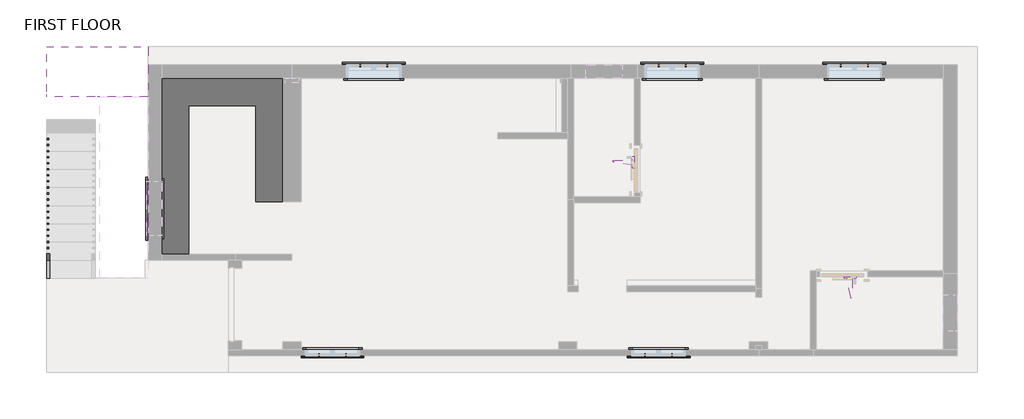
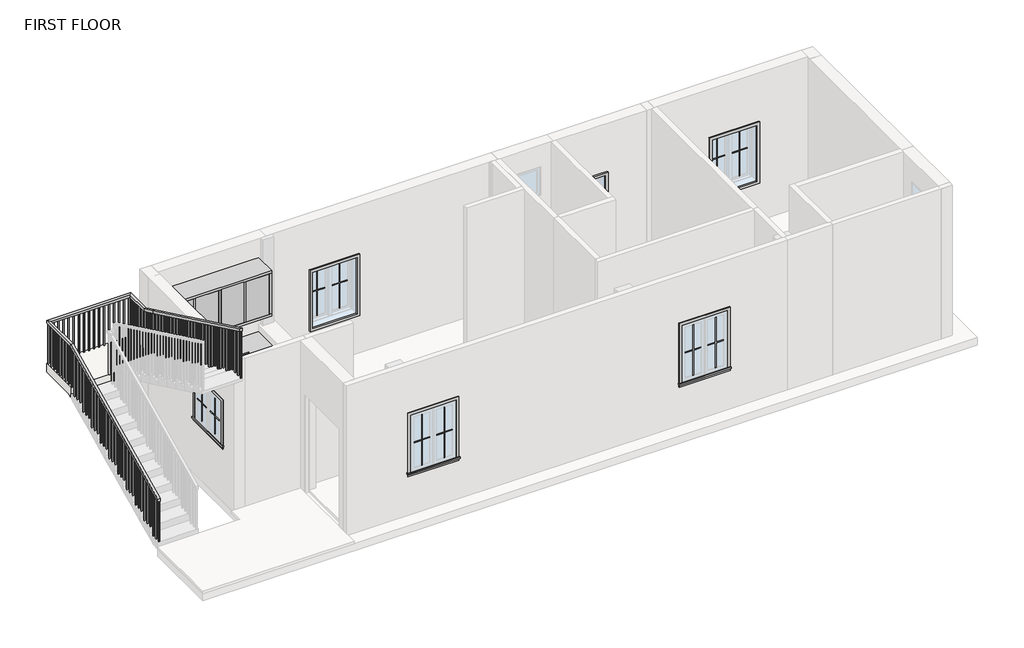
# One storey, part 3 of 3: 27 proxies, 1 railing, 1 slab.
"""IFC4 building model written with IfcOpenShell, lengths in millimetres."""

from ifc_helpers import new_model, si_unit, frame, origin, place, context, project, spatial, polyline, outline, extrude, faceted_brep, transform, mapped, element, save
from components import bel_door_closer_bel_door_closer_f210e2f3, bel_door_closer_bel_door_closer_a3520c2f, generic_models_2_generic_models_1_30118c6b, muntin_pattern_2x2_muntin_pattern_2x2_1acec82f, muntin_pattern_2x2_muntin_pattern_2x2_43d02eee, muntin_pattern_2x2_muntin_pattern_2x2_d1c6e638, muntin_pattern_2x2_muntin_pattern_2x2_37b95fb2, trim_window_exterior_flat_with_sill_e4b28ec3, trim_window_exterior_flat_with_sill_84e24481, trim_window_interior_flat_picture_frame_39ff4276, trim_window_interior_flat_picture_frame_28d4e5dc

model = new_model("IFC4")

# Units and contexts
model_context = context("Model", 3, world=origin())
ifc_project = project(units=[si_unit("LENGTHUNIT", "METRE", prefix="MILLI")], contexts=[model_context])

# Site, building, storey
site = spatial("IfcSite", under=ifc_project)
building = spatial("IfcBuilding", under=site)
storey = spatial("IfcBuildingStorey", under=building, Name="FIRST FLOOR", Elevation=3200.4)

# Proxies
placement = place(None, origin())
bel_door_closer_bel_door_closer_shape = bel_door_closer_bel_door_closer_f210e2f3(model_context)
element("IfcBuildingElementProxy", 1, Name="BEL-Door Closer : BEL-Door Closer", ObjectType="BEL-Door Closer : BEL-Door Closer", at=placement, inside=storey, context=model_context, shape_type="MappedRepresentation", body=[
    mapped(bel_door_closer_bel_door_closer_shape, transform((6826.3533773, 1546.5642852, 5345.0957985), x_axis=(-1.0, 0.0, 0.0), y_axis=(0.0, 0.0, -1.0), z_axis=(0.0, -1.0, 0.0))),
])
bel_door_closer_bel_door_closer_2_shape = bel_door_closer_bel_door_closer_a3520c2f(model_context)
element("IfcBuildingElementProxy", 2, Name="BEL-Door Closer : BEL-Door Closer", ObjectType="BEL-Door Closer : BEL-Door Closer", at=placement, inside=storey, context=model_context, shape_type="MappedRepresentation", body=[
    mapped(bel_door_closer_bel_door_closer_2_shape, transform((3460.0408773, 3211.0767852, 5345.0957985), x_axis=(0.0, -1.0, 0.0), y_axis=(0.0, 0.0, 1.0), z_axis=(-1.0, 0.0, 0.0))),
])
generic_models_2_generic_models_1_shape = generic_models_2_generic_models_1_30118c6b(model_context)
element("IfcBuildingElementProxy", 3, Name="Generic Models 2 : Generic Models 1", ObjectType="Generic Models 2 : Generic Models 1", at=placement, inside=storey, context=model_context, shape_type="MappedRepresentation", body=[
    mapped(generic_models_2_generic_models_1_shape, transform((0.0, 0.0, 0.0), x_axis=(1.0, 0.0, 0.0), y_axis=(0.0, 1.0, 0.0), z_axis=(0.0, 0.0, 1.0))),
])
muntin_pattern_2x2_muntin_pattern_2x2_shape = muntin_pattern_2x2_muntin_pattern_2x2_1acec82f(model_context)
element("IfcBuildingElementProxy", 4, Name="Muntin Pattern_2x2 : Muntin Pattern_2x2", ObjectType="Muntin Pattern_2x2 : Muntin Pattern_2x2", at=placement, inside=storey, context=model_context, shape_type="MappedRepresentation", body=[
    mapped(muntin_pattern_2x2_muntin_pattern_2x2_shape, transform((-1135.7716227, 5093.0392852, 4184.65), x_axis=(1.0, 0.0, 0.0), y_axis=(0.0, 1.0, 0.0), z_axis=(0.0, 0.0, 1.0))),
])
element("IfcBuildingElementProxy", 5, Name="Muntin Pattern_2x2 : Muntin Pattern_2x2", ObjectType="Muntin Pattern_2x2 : Muntin Pattern_2x2", at=placement, inside=storey, context=model_context, shape_type="MappedRepresentation", body=[
    mapped(muntin_pattern_2x2_muntin_pattern_2x2_shape, transform((3868.0283773, 5093.0392852, 4184.65), x_axis=(1.0, 0.0, 0.0), y_axis=(0.0, 1.0, 0.0), z_axis=(0.0, 0.0, 1.0))),
])
element("IfcBuildingElementProxy", 6, Name="Muntin Pattern_2x2 : Muntin Pattern_2x2", ObjectType="Muntin Pattern_2x2 : Muntin Pattern_2x2", at=placement, inside=storey, context=model_context, shape_type="MappedRepresentation", body=[
    mapped(muntin_pattern_2x2_muntin_pattern_2x2_shape, transform((6922.3783773, 5093.0392852, 4184.65), x_axis=(1.0, 0.0, 0.0), y_axis=(0.0, 1.0, 0.0), z_axis=(0.0, 0.0, 1.0))),
])
element("IfcBuildingElementProxy", 7, Name="Muntin Pattern_2x2 : Muntin Pattern_2x2", ObjectType="Muntin Pattern_2x2 : Muntin Pattern_2x2", at=placement, inside=storey, context=model_context, shape_type="MappedRepresentation", body=[
    mapped(muntin_pattern_2x2_muntin_pattern_2x2_shape, transform((4093.4533773, 235.2892852, 4184.65), x_axis=(-1.0, 0.0, 0.0), y_axis=(0.0, -1.0, 0.0), z_axis=(0.0, 0.0, 1.0))),
])
element("IfcBuildingElementProxy", 8, Name="Muntin Pattern_2x2 : Muntin Pattern_2x2", ObjectType="Muntin Pattern_2x2 : Muntin Pattern_2x2", at=placement, inside=storey, context=model_context, shape_type="MappedRepresentation", body=[
    mapped(muntin_pattern_2x2_muntin_pattern_2x2_shape, transform((-1373.8966227, 235.2892852, 4184.65), x_axis=(-1.0, 0.0, 0.0), y_axis=(0.0, -1.0, 0.0), z_axis=(0.0, 0.0, 1.0))),
])
muntin_pattern_2x2_muntin_pattern_2x2_2_shape = muntin_pattern_2x2_muntin_pattern_2x2_43d02eee(model_context)
element("IfcBuildingElementProxy", 9, Name="Muntin Pattern_2x2 : Muntin Pattern_2x2", ObjectType="Muntin Pattern_2x2 : Muntin Pattern_2x2", at=placement, inside=storey, context=model_context, shape_type="MappedRepresentation", body=[
    mapped(muntin_pattern_2x2_muntin_pattern_2x2_2_shape, transform((-681.7466227, 5093.0392852, 4184.65), x_axis=(-1.0, 0.0, 0.0), y_axis=(0.0, -1.0, 0.0), z_axis=(0.0, 0.0, 1.0))),
])
element("IfcBuildingElementProxy", 10, Name="Muntin Pattern_2x2 : Muntin Pattern_2x2", ObjectType="Muntin Pattern_2x2 : Muntin Pattern_2x2", at=placement, inside=storey, context=model_context, shape_type="MappedRepresentation", body=[
    mapped(muntin_pattern_2x2_muntin_pattern_2x2_2_shape, transform((4322.0533773, 5093.0392852, 4184.65), x_axis=(-1.0, 0.0, 0.0), y_axis=(0.0, -1.0, 0.0), z_axis=(0.0, 0.0, 1.0))),
])
element("IfcBuildingElementProxy", 11, Name="Muntin Pattern_2x2 : Muntin Pattern_2x2", ObjectType="Muntin Pattern_2x2 : Muntin Pattern_2x2", at=placement, inside=storey, context=model_context, shape_type="MappedRepresentation", body=[
    mapped(muntin_pattern_2x2_muntin_pattern_2x2_2_shape, transform((7376.4033773, 5093.0392852, 4184.65), x_axis=(-1.0, 0.0, 0.0), y_axis=(0.0, -1.0, 0.0), z_axis=(0.0, 0.0, 1.0))),
])
element("IfcBuildingElementProxy", 12, Name="Muntin Pattern_2x2 : Muntin Pattern_2x2", ObjectType="Muntin Pattern_2x2 : Muntin Pattern_2x2", at=placement, inside=storey, context=model_context, shape_type="MappedRepresentation", body=[
    mapped(muntin_pattern_2x2_muntin_pattern_2x2_2_shape, transform((3639.4283773, 235.2892852, 4184.65), x_axis=(1.0, 0.0, 0.0), y_axis=(0.0, 1.0, 0.0), z_axis=(0.0, 0.0, 1.0))),
])
element("IfcBuildingElementProxy", 13, Name="Muntin Pattern_2x2 : Muntin Pattern_2x2", ObjectType="Muntin Pattern_2x2 : Muntin Pattern_2x2", at=placement, inside=storey, context=model_context, shape_type="MappedRepresentation", body=[
    mapped(muntin_pattern_2x2_muntin_pattern_2x2_2_shape, transform((-1827.9216227, 235.2892852, 4184.65), x_axis=(1.0, 0.0, 0.0), y_axis=(0.0, 1.0, 0.0), z_axis=(0.0, 0.0, 1.0))),
])
muntin_pattern_2x2_muntin_pattern_2x2_3_shape = muntin_pattern_2x2_muntin_pattern_2x2_d1c6e638(model_context)
element("IfcBuildingElementProxy", 14, Name="Muntin Pattern_2x2 : Muntin Pattern_2x2", ObjectType="Muntin Pattern_2x2 : Muntin Pattern_2x2", at=placement, inside=storey, context=model_context, shape_type="MappedRepresentation", body=[
    mapped(muntin_pattern_2x2_muntin_pattern_2x2_3_shape, transform((-4683.8341227, 2462.5517852, 4489.45), x_axis=(0.0, 1.0, 0.0), y_axis=(-1.0, 0.0, 0.0), z_axis=(0.0, 0.0, 1.0))),
])
muntin_pattern_2x2_muntin_pattern_2x2_4_shape = muntin_pattern_2x2_muntin_pattern_2x2_37b95fb2(model_context)
element("IfcBuildingElementProxy", 15, Name="Muntin Pattern_2x2 : Muntin Pattern_2x2", ObjectType="Muntin Pattern_2x2 : Muntin Pattern_2x2", at=placement, inside=storey, context=model_context, shape_type="MappedRepresentation", body=[
    mapped(muntin_pattern_2x2_muntin_pattern_2x2_4_shape, transform((-4683.8341227, 2916.5767852, 4489.45), x_axis=(0.0, -1.0, 0.0), y_axis=(1.0, 0.0, 0.0), z_axis=(0.0, 0.0, 1.0))),
])
trim_window_exterior_flat_with_sill_shape = trim_window_exterior_flat_with_sill_e4b28ec3(model_context)
element("IfcBuildingElementProxy", 16, Name="Trim-Window-Exterior-Flat : with Sill", ObjectType="Trim-Window-Exterior-Flat : with Sill", at=placement, inside=storey, context=model_context, shape_type="MappedRepresentation", body=[
    mapped(trim_window_exterior_flat_with_sill_shape, transform((-908.7591227, 5102.5642852, 5334.0), x_axis=(-1.0, 0.0, 0.0), y_axis=(0.0, 0.0, 1.0), z_axis=(0.0, 1.0, 0.0))),
])
element("IfcBuildingElementProxy", 17, Name="Trim-Window-Exterior-Flat : with Sill", ObjectType="Trim-Window-Exterior-Flat : with Sill", at=placement, inside=storey, context=model_context, shape_type="MappedRepresentation", body=[
    mapped(trim_window_exterior_flat_with_sill_shape, transform((4095.0408773, 5102.5642852, 5334.0), x_axis=(-1.0, 0.0, 0.0), y_axis=(0.0, 0.0, 1.0), z_axis=(0.0, 1.0, 0.0))),
])
element("IfcBuildingElementProxy", 18, Name="Trim-Window-Exterior-Flat : with Sill", ObjectType="Trim-Window-Exterior-Flat : with Sill", at=placement, inside=storey, context=model_context, shape_type="MappedRepresentation", body=[
    mapped(trim_window_exterior_flat_with_sill_shape, transform((7149.3908773, 5102.5642852, 5334.0), x_axis=(-1.0, 0.0, 0.0), y_axis=(0.0, 0.0, 1.0), z_axis=(0.0, 1.0, 0.0))),
])
element("IfcBuildingElementProxy", 19, Name="Trim-Window-Exterior-Flat : with Sill", ObjectType="Trim-Window-Exterior-Flat : with Sill", at=placement, inside=storey, context=model_context, shape_type="MappedRepresentation", body=[
    mapped(trim_window_exterior_flat_with_sill_shape, transform((3866.4408773, 225.7642852, 5334.0), x_axis=(1.0, 0.0, 0.0), y_axis=(0.0, 0.0, 1.0), z_axis=(0.0, -1.0, 0.0))),
])
element("IfcBuildingElementProxy", 20, Name="Trim-Window-Exterior-Flat : with Sill", ObjectType="Trim-Window-Exterior-Flat : with Sill", at=placement, inside=storey, context=model_context, shape_type="MappedRepresentation", body=[
    mapped(trim_window_exterior_flat_with_sill_shape, transform((-1600.9091227, 225.7642852, 5334.0), x_axis=(1.0, 0.0, 0.0), y_axis=(0.0, 0.0, 1.0), z_axis=(0.0, -1.0, 0.0))),
])
trim_window_exterior_flat_with_sill_2_shape = trim_window_exterior_flat_with_sill_84e24481(model_context)
element("IfcBuildingElementProxy", 21, Name="Trim-Window-Exterior-Flat : with Sill", ObjectType="Trim-Window-Exterior-Flat : with Sill", at=placement, inside=storey, context=model_context, shape_type="MappedRepresentation", body=[
    mapped(trim_window_exterior_flat_with_sill_2_shape, transform((-4693.3591227, 2689.5642852, 5334.0), x_axis=(0.0, -1.0, 0.0), y_axis=(0.0, 0.0, 1.0), z_axis=(-1.0, 0.0, 0.0))),
])
trim_window_interior_flat_picture_frame_shape = trim_window_interior_flat_picture_frame_39ff4276(model_context)
element("IfcBuildingElementProxy", 22, Name="Trim-Window-Interior-Flat : Picture Frame", ObjectType="Trim-Window-Interior-Flat : Picture Frame", at=placement, inside=storey, context=model_context, shape_type="MappedRepresentation", body=[
    mapped(trim_window_interior_flat_picture_frame_shape, transform((-908.7591227, 4873.9642852, 5334.0), x_axis=(1.0, 0.0, 0.0), y_axis=(0.0, 0.0, 1.0), z_axis=(0.0, -1.0, 0.0))),
])
element("IfcBuildingElementProxy", 23, Name="Trim-Window-Interior-Flat : Picture Frame", ObjectType="Trim-Window-Interior-Flat : Picture Frame", at=placement, inside=storey, context=model_context, shape_type="MappedRepresentation", body=[
    mapped(trim_window_interior_flat_picture_frame_shape, transform((4095.0408773, 4873.9642852, 5334.0), x_axis=(1.0, 0.0, 0.0), y_axis=(0.0, 0.0, 1.0), z_axis=(0.0, -1.0, 0.0))),
])
element("IfcBuildingElementProxy", 24, Name="Trim-Window-Interior-Flat : Picture Frame", ObjectType="Trim-Window-Interior-Flat : Picture Frame", at=placement, inside=storey, context=model_context, shape_type="MappedRepresentation", body=[
    mapped(trim_window_interior_flat_picture_frame_shape, transform((7149.3908773, 4873.9642852, 5334.0), x_axis=(1.0, 0.0, 0.0), y_axis=(0.0, 0.0, 1.0), z_axis=(0.0, -1.0, 0.0))),
])
element("IfcBuildingElementProxy", 25, Name="Trim-Window-Interior-Flat : Picture Frame", ObjectType="Trim-Window-Interior-Flat : Picture Frame", at=placement, inside=storey, context=model_context, shape_type="MappedRepresentation", body=[
    mapped(trim_window_interior_flat_picture_frame_shape, transform((3866.4408773, 327.3642852, 5334.0), x_axis=(-1.0, 0.0, 0.0), y_axis=(0.0, 0.0, 1.0), z_axis=(0.0, 1.0, 0.0))),
])
element("IfcBuildingElementProxy", 26, Name="Trim-Window-Interior-Flat : Picture Frame", ObjectType="Trim-Window-Interior-Flat : Picture Frame", at=placement, inside=storey, context=model_context, shape_type="MappedRepresentation", body=[
    mapped(trim_window_interior_flat_picture_frame_shape, transform((-1600.9091227, 327.3642852, 5334.0), x_axis=(-1.0, 0.0, 0.0), y_axis=(0.0, 0.0, 1.0), z_axis=(0.0, 1.0, 0.0))),
])
trim_window_interior_flat_picture_frame_2_shape = trim_window_interior_flat_picture_frame_28d4e5dc(model_context)
element("IfcBuildingElementProxy", 27, Name="Trim-Window-Interior-Flat : Picture Frame", ObjectType="Trim-Window-Interior-Flat : Picture Frame", at=placement, inside=storey, context=model_context, shape_type="MappedRepresentation", body=[
    mapped(trim_window_interior_flat_picture_frame_2_shape, transform((-4464.7591227, 2689.5642852, 5334.0), x_axis=(0.0, 1.0, 0.0), y_axis=(0.0, 0.0, 1.0), z_axis=(1.0, 0.0, 0.0))),
])

# Railing
element("IfcRailing", 28, ObjectType="Handrail - Rectangular", at=placement, inside=storey, context=model_context, shape_type="SolidModel", body=[
    faceted_brep([(-6395.1591227, 1521.1642852, 4260.2727273), (-6395.1591227, 1521.1642852, 4203.9834559), (-6344.3591227, 1521.1642852, 4203.9834559), (-6344.3591227, 1521.1642852, 4260.2727273), (-6395.1591227, 4569.1642852, 5715.0), (-6395.1591227, 4580.6656156, 5664.2), (-6344.3591227, 4580.6656156, 5664.2), (-6344.3591227, 4569.1642852, 5715.0), (-6395.1591227, 5407.3642852, 5715.0), (-6395.1591227, 5407.3642852, 5664.2), (-6344.3591227, 5356.5642852, 5664.2), (-6344.3591227, 5356.5642852, 5715.0), (-4693.3591227, 5407.3642852, 5715.0), (-4693.3591227, 5407.3642852, 5664.2), (-4744.1591227, 5356.5642852, 5664.2), (-4744.1591227, 5356.5642852, 5715.0), (-4693.3591227, 4873.9642852, 5715.0), (-4693.3591227, 4862.4629548, 5664.2), (-4744.1591227, 4862.4629548, 5664.2), (-4744.1591227, 4873.9642852, 5715.0), (-4693.3591227, 4569.1642852, 5860.4727273), (-4693.3591227, 4547.2832222, 5814.6266906), (-4744.1591227, 4547.2832222, 5814.6266906), (-4744.1591227, 4569.1642852, 5860.4727273), (-4693.3591227, 1521.1642852, 7315.2), (-4744.1591227, 1521.1642852, 7315.2), (-4744.1591227, 1521.1642852, 7258.9107287), (-4693.3591227, 1521.1642852, 7258.9107287)], [[[0, 1, 2, 3]], [[1, 0, 4, 5]], [[2, 1, 5, 6]], [[3, 2, 6, 7]], [[0, 3, 7, 4]], [[5, 4, 8, 9]], [[6, 5, 9, 10]], [[7, 6, 10, 11]], [[4, 7, 11, 8]], [[9, 8, 12, 13]], [[10, 9, 13, 14]], [[11, 10, 14, 15]], [[8, 11, 15, 12]], [[13, 12, 16, 17]], [[14, 13, 17, 18]], [[15, 14, 18, 19]], [[12, 15, 19, 16]], [[17, 16, 20, 21]], [[18, 17, 21, 22]], [[19, 18, 22, 23]], [[16, 19, 23, 20]], [[24, 25, 26, 27]], [[21, 20, 24, 27]], [[22, 21, 27, 26]], [[23, 22, 26, 25]], [[20, 23, 25, 24]]]),
    extrude(outline(polyline([(1632.2892852, 7205.8737969), (1632.2892852, 6255.3272727), (1613.2392852, 6255.3272727), (1613.2392852, 7214.9658423), (1632.2892852, 7205.8737969)])), frame((-4728.2841227, 0.0, 0.0), z_axis=(1.0, 0.0, 0.0), x_axis=(0.0, 1.0, 0.0)), (0.0, 0.0, 1.0), 19.05),
    extrude(outline(polyline([(1733.8892852, 7157.3828878), (1733.8892852, 6255.3272727), (1714.8392852, 6255.3272727), (1714.8392852, 7166.4749332), (1733.8892852, 7157.3828878)])), frame((-4728.2841227, 0.0, 0.0), z_axis=(1.0, 0.0, 0.0), x_axis=(0.0, 1.0, 0.0)), (0.0, 0.0, 1.0), 19.05),
    extrude(outline(polyline([(1835.4892852, 7108.8919787), (1835.4892852, 6255.3272727), (1816.4392852, 6255.3272727), (1816.4392852, 7117.9840241), (1835.4892852, 7108.8919787)])), frame((-4728.2841227, 0.0, 0.0), z_axis=(1.0, 0.0, 0.0), x_axis=(0.0, 1.0, 0.0)), (0.0, 0.0, 1.0), 19.05),
    extrude(outline(polyline([(1937.0892852, 7060.4010696), (1937.0892852, 6109.8545455), (1918.0392852, 6109.8545455), (1918.0392852, 7069.493115), (1937.0892852, 7060.4010696)])), frame((-4728.2841227, 0.0, 0.0), z_axis=(1.0, 0.0, 0.0), x_axis=(0.0, 1.0, 0.0)), (0.0, 0.0, 1.0), 19.05),
    extrude(outline(polyline([(2038.6892852, 7011.9101605), (2038.6892852, 6109.8545455), (2019.6392852, 6109.8545455), (2019.6392852, 7021.0022059), (2038.6892852, 7011.9101605)])), frame((-4728.2841227, 0.0, 0.0), z_axis=(1.0, 0.0, 0.0), x_axis=(0.0, 1.0, 0.0)), (0.0, 0.0, 1.0), 19.05),
    extrude(outline(polyline([(2140.2892852, 6963.4192514), (2140.2892852, 6109.8545455), (2121.2392852, 6109.8545455), (2121.2392852, 6972.5112969), (2140.2892852, 6963.4192514)])), frame((-4728.2841227, 0.0, 0.0), z_axis=(1.0, 0.0, 0.0), x_axis=(0.0, 1.0, 0.0)), (0.0, 0.0, 1.0), 19.05),
    extrude(outline(polyline([(2241.8892852, 6914.9283423), (2241.8892852, 5964.3818182), (2222.8392852, 5964.3818182), (2222.8392852, 6924.0203878), (2241.8892852, 6914.9283423)])), frame((-4728.2841227, 0.0, 0.0), z_axis=(1.0, 0.0, 0.0), x_axis=(0.0, 1.0, 0.0)), (0.0, 0.0, 1.0), 19.05),
    extrude(outline(polyline([(2343.4892852, 6866.4374332), (2343.4892852, 5964.3818182), (2324.4392852, 5964.3818182), (2324.4392852, 6875.5294787), (2343.4892852, 6866.4374332)])), frame((-4728.2841227, 0.0, 0.0), z_axis=(1.0, 0.0, 0.0), x_axis=(0.0, 1.0, 0.0)), (0.0, 0.0, 1.0), 19.05),
    extrude(outline(polyline([(2445.0892852, 6817.9465241), (2445.0892852, 5964.3818182), (2426.0392852, 5964.3818182), (2426.0392852, 6827.0385696), (2445.0892852, 6817.9465241)])), frame((-4728.2841227, 0.0, 0.0), z_axis=(1.0, 0.0, 0.0), x_axis=(0.0, 1.0, 0.0)), (0.0, 0.0, 1.0), 19.05),
    extrude(outline(polyline([(2546.6892852, 6769.455615), (2546.6892852, 5818.9090909), (2527.6392852, 5818.9090909), (2527.6392852, 6778.5476605), (2546.6892852, 6769.455615)])), frame((-4728.2841227, 0.0, 0.0), z_axis=(1.0, 0.0, 0.0), x_axis=(0.0, 1.0, 0.0)), (0.0, 0.0, 1.0), 19.05),
    extrude(outline(polyline([(2648.2892852, 6720.9647059), (2648.2892852, 5818.9090909), (2629.2392852, 5818.9090909), (2629.2392852, 6730.0567514), (2648.2892852, 6720.9647059)])), frame((-4728.2841227, 0.0, 0.0), z_axis=(1.0, 0.0, 0.0), x_axis=(0.0, 1.0, 0.0)), (0.0, 0.0, 1.0), 19.05),
    extrude(outline(polyline([(2749.8892852, 6672.4737969), (2749.8892852, 5818.9090909), (2730.8392852, 5818.9090909), (2730.8392852, 6681.5658423), (2749.8892852, 6672.4737969)])), frame((-4728.2841227, 0.0, 0.0), z_axis=(1.0, 0.0, 0.0), x_axis=(0.0, 1.0, 0.0)), (0.0, 0.0, 1.0), 19.05),
    extrude(outline(polyline([(2851.4892852, 6623.9828878), (2851.4892852, 5673.4363636), (2832.4392852, 5673.4363636), (2832.4392852, 6633.0749332), (2851.4892852, 6623.9828878)])), frame((-4728.2841227, 0.0, 0.0), z_axis=(1.0, 0.0, 0.0), x_axis=(0.0, 1.0, 0.0)), (0.0, 0.0, 1.0), 19.05),
    extrude(outline(polyline([(2953.0892852, 6575.4919787), (2953.0892852, 5673.4363636), (2934.0392852, 5673.4363636), (2934.0392852, 6584.5840241), (2953.0892852, 6575.4919787)])), frame((-4728.2841227, 0.0, 0.0), z_axis=(1.0, 0.0, 0.0), x_axis=(0.0, 1.0, 0.0)), (0.0, 0.0, 1.0), 19.05),
    extrude(outline(polyline([(3054.6892852, 6527.0010696), (3054.6892852, 5673.4363636), (3035.6392852, 5673.4363636), (3035.6392852, 6536.093115), (3054.6892852, 6527.0010696)])), frame((-4728.2841227, 0.0, 0.0), z_axis=(1.0, 0.0, 0.0), x_axis=(0.0, 1.0, 0.0)), (0.0, 0.0, 1.0), 19.05),
    extrude(outline(polyline([(3156.2892852, 6478.5101605), (3156.2892852, 5527.9636364), (3137.2392852, 5527.9636364), (3137.2392852, 6487.6022059), (3156.2892852, 6478.5101605)])), frame((-4728.2841227, 0.0, 0.0), z_axis=(1.0, 0.0, 0.0), x_axis=(0.0, 1.0, 0.0)), (0.0, 0.0, 1.0), 19.05),
    extrude(outline(polyline([(3257.8892852, 6430.0192514), (3257.8892852, 5527.9636364), (3238.8392852, 5527.9636364), (3238.8392852, 6439.1112969), (3257.8892852, 6430.0192514)])), frame((-4728.2841227, 0.0, 0.0), z_axis=(1.0, 0.0, 0.0), x_axis=(0.0, 1.0, 0.0)), (0.0, 0.0, 1.0), 19.05),
    extrude(outline(polyline([(3359.4892852, 6381.5283423), (3359.4892852, 5527.9636364), (3340.4392852, 5527.9636364), (3340.4392852, 6390.6203878), (3359.4892852, 6381.5283423)])), frame((-4728.2841227, 0.0, 0.0), z_axis=(1.0, 0.0, 0.0), x_axis=(0.0, 1.0, 0.0)), (0.0, 0.0, 1.0), 19.05),
    extrude(outline(polyline([(3461.0892852, 6333.0374332), (3461.0892852, 5382.4909091), (3442.0392852, 5382.4909091), (3442.0392852, 6342.1294787), (3461.0892852, 6333.0374332)])), frame((-4728.2841227, 0.0, 0.0), z_axis=(1.0, 0.0, 0.0), x_axis=(0.0, 1.0, 0.0)), (0.0, 0.0, 1.0), 19.05),
    extrude(outline(polyline([(3562.6892852, 6284.5465241), (3562.6892852, 5382.4909091), (3543.6392852, 5382.4909091), (3543.6392852, 6293.6385696), (3562.6892852, 6284.5465241)])), frame((-4728.2841227, 0.0, 0.0), z_axis=(1.0, 0.0, 0.0), x_axis=(0.0, 1.0, 0.0)), (0.0, 0.0, 1.0), 19.05),
    extrude(outline(polyline([(3664.2892852, 6236.055615), (3664.2892852, 5382.4909091), (3645.2392852, 5382.4909091), (3645.2392852, 6245.1476605), (3664.2892852, 6236.055615)])), frame((-4728.2841227, 0.0, 0.0), z_axis=(1.0, 0.0, 0.0), x_axis=(0.0, 1.0, 0.0)), (0.0, 0.0, 1.0), 19.05),
    extrude(outline(polyline([(3765.8892852, 6187.5647059), (3765.8892852, 5237.0181818), (3746.8392852, 5237.0181818), (3746.8392852, 6196.6567514), (3765.8892852, 6187.5647059)])), frame((-4728.2841227, 0.0, 0.0), z_axis=(1.0, 0.0, 0.0), x_axis=(0.0, 1.0, 0.0)), (0.0, 0.0, 1.0), 19.05),
    extrude(outline(polyline([(3867.4892852, 6139.0737969), (3867.4892852, 5237.0181818), (3848.4392852, 5237.0181818), (3848.4392852, 6148.1658423), (3867.4892852, 6139.0737969)])), frame((-4728.2841227, 0.0, 0.0), z_axis=(1.0, 0.0, 0.0), x_axis=(0.0, 1.0, 0.0)), (0.0, 0.0, 1.0), 19.05),
    extrude(outline(polyline([(3969.0892852, 6090.5828878), (3969.0892852, 5237.0181818), (3950.0392852, 5237.0181818), (3950.0392852, 6099.6749332), (3969.0892852, 6090.5828878)])), frame((-4728.2841227, 0.0, 0.0), z_axis=(1.0, 0.0, 0.0), x_axis=(0.0, 1.0, 0.0)), (0.0, 0.0, 1.0), 19.05),
    extrude(outline(polyline([(4070.6892852, 6042.0919787), (4070.6892852, 5091.5454545), (4051.6392852, 5091.5454545), (4051.6392852, 6051.1840241), (4070.6892852, 6042.0919787)])), frame((-4728.2841227, 0.0, 0.0), z_axis=(1.0, 0.0, 0.0), x_axis=(0.0, 1.0, 0.0)), (0.0, 0.0, 1.0), 19.05),
    extrude(outline(polyline([(4172.2892852, 5993.6010696), (4172.2892852, 5091.5454545), (4153.2392852, 5091.5454545), (4153.2392852, 6002.693115), (4172.2892852, 5993.6010696)])), frame((-4728.2841227, 0.0, 0.0), z_axis=(1.0, 0.0, 0.0), x_axis=(0.0, 1.0, 0.0)), (0.0, 0.0, 1.0), 19.05),
    extrude(outline(polyline([(4273.8892852, 5945.1101605), (4273.8892852, 5091.5454545), (4254.8392852, 5091.5454545), (4254.8392852, 5954.2022059), (4273.8892852, 5945.1101605)])), frame((-4728.2841227, 0.0, 0.0), z_axis=(1.0, 0.0, 0.0), x_axis=(0.0, 1.0, 0.0)), (0.0, 0.0, 1.0), 19.05),
    extrude(outline(polyline([(4375.4892852, 5896.6192514), (4375.4892852, 4946.0727273), (4356.4392852, 4946.0727273), (4356.4392852, 5905.7112969), (4375.4892852, 5896.6192514)])), frame((-4728.2841227, 0.0, 0.0), z_axis=(1.0, 0.0, 0.0), x_axis=(0.0, 1.0, 0.0)), (0.0, 0.0, 1.0), 19.05),
    extrude(outline(polyline([(4477.0892852, 5848.1283423), (4477.0892852, 4946.0727273), (4458.0392852, 4946.0727273), (4458.0392852, 5857.2203878), (4477.0892852, 5848.1283423)])), frame((-4728.2841227, 0.0, 0.0), z_axis=(1.0, 0.0, 0.0), x_axis=(0.0, 1.0, 0.0)), (0.0, 0.0, 1.0), 19.05),
    extrude(outline(polyline([(4680.2892852, 5751.1465241), (4680.2892852, 4800.6), (4661.2392852, 4800.6), (4661.2392852, 5760.2385696), (4680.2892852, 5751.1465241)])), frame((-4728.2841227, 0.0, 0.0), z_axis=(1.0, 0.0, 0.0), x_axis=(0.0, 1.0, 0.0)), (0.0, 0.0, 1.0), 19.05),
    extrude(outline(polyline([(4781.8892852, 5702.655615), (4781.8892852, 4800.6), (4762.8392852, 4800.6), (4762.8392852, 5711.7476605), (4781.8892852, 5702.655615)])), frame((-4728.2841227, 0.0, 0.0), z_axis=(1.0, 0.0, 0.0), x_axis=(0.0, 1.0, 0.0)), (0.0, 0.0, 1.0), 19.05),
    extrude(outline(polyline([(-4709.2341227, 4883.4892852), (-4709.2341227, 4864.4392852), (-4728.2841227, 4864.4392852), (-4728.2841227, 4883.4892852), (-4709.2341227, 4883.4892852)])), frame((0.0, 0.0, 4800.6), z_axis=(0.0, 0.0, 1.0), x_axis=(1.0, 0.0, 0.0)), (0.0, 0.0, 1.0), 863.6),
    extrude(outline(polyline([(-4709.2341227, 4985.0892852), (-4709.2341227, 4966.0392852), (-4728.2841227, 4966.0392852), (-4728.2841227, 4985.0892852), (-4709.2341227, 4985.0892852)])), frame((0.0, 0.0, 4800.6), z_axis=(0.0, 0.0, 1.0), x_axis=(1.0, 0.0, 0.0)), (0.0, 0.0, 1.0), 863.6),
    extrude(outline(polyline([(-4709.2341227, 5086.6892852), (-4709.2341227, 5067.6392852), (-4728.2841227, 5067.6392852), (-4728.2841227, 5086.6892852), (-4709.2341227, 5086.6892852)])), frame((0.0, 0.0, 4800.6), z_axis=(0.0, 0.0, 1.0), x_axis=(1.0, 0.0, 0.0)), (0.0, 0.0, 1.0), 863.6),
    extrude(outline(polyline([(-4709.2341227, 5188.2892852), (-4709.2341227, 5169.2392852), (-4728.2841227, 5169.2392852), (-4728.2841227, 5188.2892852), (-4709.2341227, 5188.2892852)])), frame((0.0, 0.0, 4800.6), z_axis=(0.0, 0.0, 1.0), x_axis=(1.0, 0.0, 0.0)), (0.0, 0.0, 1.0), 863.6),
    extrude(outline(polyline([(-4709.2341227, 5289.8892852), (-4709.2341227, 5270.8392852), (-4728.2841227, 5270.8392852), (-4728.2841227, 5289.8892852), (-4709.2341227, 5289.8892852)])), frame((0.0, 0.0, 4800.6), z_axis=(0.0, 0.0, 1.0), x_axis=(1.0, 0.0, 0.0)), (0.0, 0.0, 1.0), 863.6),
    extrude(outline(polyline([(-4753.6841227, 5391.4892852), (-4734.6341227, 5391.4892852), (-4734.6341227, 5372.4392852), (-4753.6841227, 5372.4392852), (-4753.6841227, 5391.4892852)])), frame((0.0, 0.0, 4800.6), z_axis=(0.0, 0.0, 1.0), x_axis=(1.0, 0.0, 0.0)), (0.0, 0.0, 1.0), 863.6),
    extrude(outline(polyline([(-4855.2841227, 5391.4892852), (-4836.2341227, 5391.4892852), (-4836.2341227, 5372.4392852), (-4855.2841227, 5372.4392852), (-4855.2841227, 5391.4892852)])), frame((0.0, 0.0, 4800.6), z_axis=(0.0, 0.0, 1.0), x_axis=(1.0, 0.0, 0.0)), (0.0, 0.0, 1.0), 863.6),
    extrude(outline(polyline([(-4956.8841227, 5391.4892852), (-4937.8341227, 5391.4892852), (-4937.8341227, 5372.4392852), (-4956.8841227, 5372.4392852), (-4956.8841227, 5391.4892852)])), frame((0.0, 0.0, 4800.6), z_axis=(0.0, 0.0, 1.0), x_axis=(1.0, 0.0, 0.0)), (0.0, 0.0, 1.0), 863.6),
    extrude(outline(polyline([(-5058.4841227, 5391.4892852), (-5039.4341227, 5391.4892852), (-5039.4341227, 5372.4392852), (-5058.4841227, 5372.4392852), (-5058.4841227, 5391.4892852)])), frame((0.0, 0.0, 4800.6), z_axis=(0.0, 0.0, 1.0), x_axis=(1.0, 0.0, 0.0)), (0.0, 0.0, 1.0), 863.6),
    extrude(outline(polyline([(-5160.0841227, 5391.4892852), (-5141.0341227, 5391.4892852), (-5141.0341227, 5372.4392852), (-5160.0841227, 5372.4392852), (-5160.0841227, 5391.4892852)])), frame((0.0, 0.0, 4800.6), z_axis=(0.0, 0.0, 1.0), x_axis=(1.0, 0.0, 0.0)), (0.0, 0.0, 1.0), 863.6),
    extrude(outline(polyline([(-5261.6841227, 5391.4892852), (-5242.6341227, 5391.4892852), (-5242.6341227, 5372.4392852), (-5261.6841227, 5372.4392852), (-5261.6841227, 5391.4892852)])), frame((0.0, 0.0, 4800.6), z_axis=(0.0, 0.0, 1.0), x_axis=(1.0, 0.0, 0.0)), (0.0, 0.0, 1.0), 863.6),
    extrude(outline(polyline([(-5363.2841227, 5391.4892852), (-5344.2341227, 5391.4892852), (-5344.2341227, 5372.4392852), (-5363.2841227, 5372.4392852), (-5363.2841227, 5391.4892852)])), frame((0.0, 0.0, 4800.6), z_axis=(0.0, 0.0, 1.0), x_axis=(1.0, 0.0, 0.0)), (0.0, 0.0, 1.0), 863.6),
    extrude(outline(polyline([(-5464.8841227, 5391.4892852), (-5445.8341227, 5391.4892852), (-5445.8341227, 5372.4392852), (-5464.8841227, 5372.4392852), (-5464.8841227, 5391.4892852)])), frame((0.0, 0.0, 4800.6), z_axis=(0.0, 0.0, 1.0), x_axis=(1.0, 0.0, 0.0)), (0.0, 0.0, 1.0), 863.6),
    extrude(outline(polyline([(-5566.4841227, 5391.4892852), (-5547.4341227, 5391.4892852), (-5547.4341227, 5372.4392852), (-5566.4841227, 5372.4392852), (-5566.4841227, 5391.4892852)])), frame((0.0, 0.0, 4800.6), z_axis=(0.0, 0.0, 1.0), x_axis=(1.0, 0.0, 0.0)), (0.0, 0.0, 1.0), 863.6),
    extrude(outline(polyline([(-5668.0841227, 5391.4892852), (-5649.0341227, 5391.4892852), (-5649.0341227, 5372.4392852), (-5668.0841227, 5372.4392852), (-5668.0841227, 5391.4892852)])), frame((0.0, 0.0, 4800.6), z_axis=(0.0, 0.0, 1.0), x_axis=(1.0, 0.0, 0.0)), (0.0, 0.0, 1.0), 863.6),
    extrude(outline(polyline([(-5769.6841227, 5391.4892852), (-5750.6341227, 5391.4892852), (-5750.6341227, 5372.4392852), (-5769.6841227, 5372.4392852), (-5769.6841227, 5391.4892852)])), frame((0.0, 0.0, 4800.6), z_axis=(0.0, 0.0, 1.0), x_axis=(1.0, 0.0, 0.0)), (0.0, 0.0, 1.0), 863.6),
    extrude(outline(polyline([(-5871.2841227, 5391.4892852), (-5852.2341227, 5391.4892852), (-5852.2341227, 5372.4392852), (-5871.2841227, 5372.4392852), (-5871.2841227, 5391.4892852)])), frame((0.0, 0.0, 4800.6), z_axis=(0.0, 0.0, 1.0), x_axis=(1.0, 0.0, 0.0)), (0.0, 0.0, 1.0), 863.6),
    extrude(outline(polyline([(-5972.8841227, 5391.4892852), (-5953.8341227, 5391.4892852), (-5953.8341227, 5372.4392852), (-5972.8841227, 5372.4392852), (-5972.8841227, 5391.4892852)])), frame((0.0, 0.0, 4800.6), z_axis=(0.0, 0.0, 1.0), x_axis=(1.0, 0.0, 0.0)), (0.0, 0.0, 1.0), 863.6),
    extrude(outline(polyline([(-6074.4841227, 5391.4892852), (-6055.4341227, 5391.4892852), (-6055.4341227, 5372.4392852), (-6074.4841227, 5372.4392852), (-6074.4841227, 5391.4892852)])), frame((0.0, 0.0, 4800.6), z_axis=(0.0, 0.0, 1.0), x_axis=(1.0, 0.0, 0.0)), (0.0, 0.0, 1.0), 863.6),
    extrude(outline(polyline([(-6176.0841227, 5391.4892852), (-6157.0341227, 5391.4892852), (-6157.0341227, 5372.4392852), (-6176.0841227, 5372.4392852), (-6176.0841227, 5391.4892852)])), frame((0.0, 0.0, 4800.6), z_axis=(0.0, 0.0, 1.0), x_axis=(1.0, 0.0, 0.0)), (0.0, 0.0, 1.0), 863.6),
    extrude(outline(polyline([(-6277.6841227, 5391.4892852), (-6258.6341227, 5391.4892852), (-6258.6341227, 5372.4392852), (-6277.6841227, 5372.4392852), (-6277.6841227, 5391.4892852)])), frame((0.0, 0.0, 4800.6), z_axis=(0.0, 0.0, 1.0), x_axis=(1.0, 0.0, 0.0)), (0.0, 0.0, 1.0), 863.6),
    extrude(outline(polyline([(-6379.2841227, 5270.8392852), (-6379.2841227, 5289.8892852), (-6360.2341227, 5289.8892852), (-6360.2341227, 5270.8392852), (-6379.2841227, 5270.8392852)])), frame((0.0, 0.0, 4800.6), z_axis=(0.0, 0.0, 1.0), x_axis=(1.0, 0.0, 0.0)), (0.0, 0.0, 1.0), 863.6),
    extrude(outline(polyline([(-6379.2841227, 5169.2392852), (-6379.2841227, 5188.2892852), (-6360.2341227, 5188.2892852), (-6360.2341227, 5169.2392852), (-6379.2841227, 5169.2392852)])), frame((0.0, 0.0, 4800.6), z_axis=(0.0, 0.0, 1.0), x_axis=(1.0, 0.0, 0.0)), (0.0, 0.0, 1.0), 863.6),
    extrude(outline(polyline([(-6379.2841227, 5067.6392852), (-6379.2841227, 5086.6892852), (-6360.2341227, 5086.6892852), (-6360.2341227, 5067.6392852), (-6379.2841227, 5067.6392852)])), frame((0.0, 0.0, 4800.6), z_axis=(0.0, 0.0, 1.0), x_axis=(1.0, 0.0, 0.0)), (0.0, 0.0, 1.0), 863.6),
    extrude(outline(polyline([(-6379.2841227, 4966.0392852), (-6379.2841227, 4985.0892852), (-6360.2341227, 4985.0892852), (-6360.2341227, 4966.0392852), (-6379.2841227, 4966.0392852)])), frame((0.0, 0.0, 4800.6), z_axis=(0.0, 0.0, 1.0), x_axis=(1.0, 0.0, 0.0)), (0.0, 0.0, 1.0), 863.6),
    extrude(outline(polyline([(-6379.2841227, 4864.4392852), (-6379.2841227, 4883.4892852), (-6360.2341227, 4883.4892852), (-6360.2341227, 4864.4392852), (-6379.2841227, 4864.4392852)])), frame((0.0, 0.0, 4800.6), z_axis=(0.0, 0.0, 1.0), x_axis=(1.0, 0.0, 0.0)), (0.0, 0.0, 1.0), 863.6),
    extrude(outline(polyline([(-6379.2841227, 4762.8392852), (-6379.2841227, 4781.8892852), (-6360.2341227, 4781.8892852), (-6360.2341227, 4762.8392852), (-6379.2841227, 4762.8392852)])), frame((0.0, 0.0, 4800.6), z_axis=(0.0, 0.0, 1.0), x_axis=(1.0, 0.0, 0.0)), (0.0, 0.0, 1.0), 863.6),
    extrude(outline(polyline([(-6379.2841227, 4661.2392852), (-6379.2841227, 4680.2892852), (-6360.2341227, 4680.2892852), (-6360.2341227, 4661.2392852), (-6379.2841227, 4661.2392852)])), frame((0.0, 0.0, 4800.6), z_axis=(0.0, 0.0, 1.0), x_axis=(1.0, 0.0, 0.0)), (0.0, 0.0, 1.0), 863.6),
    extrude(outline(polyline([(4477.0892852, 5614.7658423), (4477.0892852, 4655.1272727), (4458.0392852, 4655.1272727), (4458.0392852, 5605.6737969), (4477.0892852, 5614.7658423)])), frame((-6379.2841227, 0.0, 0.0), z_axis=(1.0, 0.0, 0.0), x_axis=(0.0, 1.0, 0.0)), (0.0, 0.0, 1.0), 19.05),
    extrude(outline(polyline([(4375.4892852, 5566.2749332), (4375.4892852, 4655.1272727), (4356.4392852, 4655.1272727), (4356.4392852, 5557.1828878), (4375.4892852, 5566.2749332)])), frame((-6379.2841227, 0.0, 0.0), z_axis=(1.0, 0.0, 0.0), x_axis=(0.0, 1.0, 0.0)), (0.0, 0.0, 1.0), 19.05),
    extrude(outline(polyline([(4273.8892852, 5517.7840241), (4273.8892852, 4655.1272727), (4254.8392852, 4655.1272727), (4254.8392852, 5508.6919787), (4273.8892852, 5517.7840241)])), frame((-6379.2841227, 0.0, 0.0), z_axis=(1.0, 0.0, 0.0), x_axis=(0.0, 1.0, 0.0)), (0.0, 0.0, 1.0), 19.05),
    extrude(outline(polyline([(4172.2892852, 5469.293115), (4172.2892852, 4509.6545455), (4153.2392852, 4509.6545455), (4153.2392852, 5460.2010696), (4172.2892852, 5469.293115)])), frame((-6379.2841227, 0.0, 0.0), z_axis=(1.0, 0.0, 0.0), x_axis=(0.0, 1.0, 0.0)), (0.0, 0.0, 1.0), 19.05),
    extrude(outline(polyline([(4070.6892852, 5420.8022059), (4070.6892852, 4509.6545455), (4051.6392852, 4509.6545455), (4051.6392852, 5411.7101605), (4070.6892852, 5420.8022059)])), frame((-6379.2841227, 0.0, 0.0), z_axis=(1.0, 0.0, 0.0), x_axis=(0.0, 1.0, 0.0)), (0.0, 0.0, 1.0), 19.05),
    extrude(outline(polyline([(3969.0892852, 5372.3112969), (3969.0892852, 4509.6545455), (3950.0392852, 4509.6545455), (3950.0392852, 5363.2192514), (3969.0892852, 5372.3112969)])), frame((-6379.2841227, 0.0, 0.0), z_axis=(1.0, 0.0, 0.0), x_axis=(0.0, 1.0, 0.0)), (0.0, 0.0, 1.0), 19.05),
    extrude(outline(polyline([(3867.4892852, 5323.8203878), (3867.4892852, 4364.1818182), (3848.4392852, 4364.1818182), (3848.4392852, 5314.7283423), (3867.4892852, 5323.8203878)])), frame((-6379.2841227, 0.0, 0.0), z_axis=(1.0, 0.0, 0.0), x_axis=(0.0, 1.0, 0.0)), (0.0, 0.0, 1.0), 19.05),
    extrude(outline(polyline([(3765.8892852, 5275.3294787), (3765.8892852, 4364.1818182), (3746.8392852, 4364.1818182), (3746.8392852, 5266.2374332), (3765.8892852, 5275.3294787)])), frame((-6379.2841227, 0.0, 0.0), z_axis=(1.0, 0.0, 0.0), x_axis=(0.0, 1.0, 0.0)), (0.0, 0.0, 1.0), 19.05),
    extrude(outline(polyline([(3664.2892852, 5226.8385696), (3664.2892852, 4364.1818182), (3645.2392852, 4364.1818182), (3645.2392852, 5217.7465241), (3664.2892852, 5226.8385696)])), frame((-6379.2841227, 0.0, 0.0), z_axis=(1.0, 0.0, 0.0), x_axis=(0.0, 1.0, 0.0)), (0.0, 0.0, 1.0), 19.05),
    extrude(outline(polyline([(3562.6892852, 5178.3476605), (3562.6892852, 4218.7090909), (3543.6392852, 4218.7090909), (3543.6392852, 5169.255615), (3562.6892852, 5178.3476605)])), frame((-6379.2841227, 0.0, 0.0), z_axis=(1.0, 0.0, 0.0), x_axis=(0.0, 1.0, 0.0)), (0.0, 0.0, 1.0), 19.05),
    extrude(outline(polyline([(3461.0892852, 5129.8567514), (3461.0892852, 4218.7090909), (3442.0392852, 4218.7090909), (3442.0392852, 5120.7647059), (3461.0892852, 5129.8567514)])), frame((-6379.2841227, 0.0, 0.0), z_axis=(1.0, 0.0, 0.0), x_axis=(0.0, 1.0, 0.0)), (0.0, 0.0, 1.0), 19.05),
    extrude(outline(polyline([(3359.4892852, 5081.3658423), (3359.4892852, 4218.7090909), (3340.4392852, 4218.7090909), (3340.4392852, 5072.2737969), (3359.4892852, 5081.3658423)])), frame((-6379.2841227, 0.0, 0.0), z_axis=(1.0, 0.0, 0.0), x_axis=(0.0, 1.0, 0.0)), (0.0, 0.0, 1.0), 19.05),
    extrude(outline(polyline([(3257.8892852, 5032.8749332), (3257.8892852, 4073.2363636), (3238.8392852, 4073.2363636), (3238.8392852, 5023.7828878), (3257.8892852, 5032.8749332)])), frame((-6379.2841227, 0.0, 0.0), z_axis=(1.0, 0.0, 0.0), x_axis=(0.0, 1.0, 0.0)), (0.0, 0.0, 1.0), 19.05),
    extrude(outline(polyline([(3156.2892852, 4984.3840241), (3156.2892852, 4073.2363636), (3137.2392852, 4073.2363636), (3137.2392852, 4975.2919787), (3156.2892852, 4984.3840241)])), frame((-6379.2841227, 0.0, 0.0), z_axis=(1.0, 0.0, 0.0), x_axis=(0.0, 1.0, 0.0)), (0.0, 0.0, 1.0), 19.05),
    extrude(outline(polyline([(3054.6892852, 4935.893115), (3054.6892852, 4073.2363636), (3035.6392852, 4073.2363636), (3035.6392852, 4926.8010696), (3054.6892852, 4935.893115)])), frame((-6379.2841227, 0.0, 0.0), z_axis=(1.0, 0.0, 0.0), x_axis=(0.0, 1.0, 0.0)), (0.0, 0.0, 1.0), 19.05),
    extrude(outline(polyline([(2953.0892852, 4887.4022059), (2953.0892852, 3927.7636364), (2934.0392852, 3927.7636364), (2934.0392852, 4878.3101605), (2953.0892852, 4887.4022059)])), frame((-6379.2841227, 0.0, 0.0), z_axis=(1.0, 0.0, 0.0), x_axis=(0.0, 1.0, 0.0)), (0.0, 0.0, 1.0), 19.05),
    extrude(outline(polyline([(2851.4892852, 4838.9112969), (2851.4892852, 3927.7636364), (2832.4392852, 3927.7636364), (2832.4392852, 4829.8192514), (2851.4892852, 4838.9112969)])), frame((-6379.2841227, 0.0, 0.0), z_axis=(1.0, 0.0, 0.0), x_axis=(0.0, 1.0, 0.0)), (0.0, 0.0, 1.0), 19.05),
    extrude(outline(polyline([(2749.8892852, 4790.4203878), (2749.8892852, 3927.7636364), (2730.8392852, 3927.7636364), (2730.8392852, 4781.3283423), (2749.8892852, 4790.4203878)])), frame((-6379.2841227, 0.0, 0.0), z_axis=(1.0, 0.0, 0.0), x_axis=(0.0, 1.0, 0.0)), (0.0, 0.0, 1.0), 19.05),
    extrude(outline(polyline([(2648.2892852, 4741.9294787), (2648.2892852, 3782.2909091), (2629.2392852, 3782.2909091), (2629.2392852, 4732.8374332), (2648.2892852, 4741.9294787)])), frame((-6379.2841227, 0.0, 0.0), z_axis=(1.0, 0.0, 0.0), x_axis=(0.0, 1.0, 0.0)), (0.0, 0.0, 1.0), 19.05),
    extrude(outline(polyline([(2546.6892852, 4693.4385696), (2546.6892852, 3782.2909091), (2527.6392852, 3782.2909091), (2527.6392852, 4684.3465241), (2546.6892852, 4693.4385696)])), frame((-6379.2841227, 0.0, 0.0), z_axis=(1.0, 0.0, 0.0), x_axis=(0.0, 1.0, 0.0)), (0.0, 0.0, 1.0), 19.05),
    extrude(outline(polyline([(2445.0892852, 4644.9476605), (2445.0892852, 3782.2909091), (2426.0392852, 3782.2909091), (2426.0392852, 4635.855615), (2445.0892852, 4644.9476605)])), frame((-6379.2841227, 0.0, 0.0), z_axis=(1.0, 0.0, 0.0), x_axis=(0.0, 1.0, 0.0)), (0.0, 0.0, 1.0), 19.05),
    extrude(outline(polyline([(2343.4892852, 4596.4567514), (2343.4892852, 3636.8181818), (2324.4392852, 3636.8181818), (2324.4392852, 4587.3647059), (2343.4892852, 4596.4567514)])), frame((-6379.2841227, 0.0, 0.0), z_axis=(1.0, 0.0, 0.0), x_axis=(0.0, 1.0, 0.0)), (0.0, 0.0, 1.0), 19.05),
    extrude(outline(polyline([(2241.8892852, 4547.9658423), (2241.8892852, 3636.8181818), (2222.8392852, 3636.8181818), (2222.8392852, 4538.8737969), (2241.8892852, 4547.9658423)])), frame((-6379.2841227, 0.0, 0.0), z_axis=(1.0, 0.0, 0.0), x_axis=(0.0, 1.0, 0.0)), (0.0, 0.0, 1.0), 19.05),
    extrude(outline(polyline([(2140.2892852, 4499.4749332), (2140.2892852, 3636.8181818), (2121.2392852, 3636.8181818), (2121.2392852, 4490.3828878), (2140.2892852, 4499.4749332)])), frame((-6379.2841227, 0.0, 0.0), z_axis=(1.0, 0.0, 0.0), x_axis=(0.0, 1.0, 0.0)), (0.0, 0.0, 1.0), 19.05),
    extrude(outline(polyline([(2038.6892852, 4450.9840241), (2038.6892852, 3491.3454545), (2019.6392852, 3491.3454545), (2019.6392852, 4441.8919787), (2038.6892852, 4450.9840241)])), frame((-6379.2841227, 0.0, 0.0), z_axis=(1.0, 0.0, 0.0), x_axis=(0.0, 1.0, 0.0)), (0.0, 0.0, 1.0), 19.05),
    extrude(outline(polyline([(1937.0892852, 4402.493115), (1937.0892852, 3491.3454545), (1918.0392852, 3491.3454545), (1918.0392852, 4393.4010696), (1937.0892852, 4402.493115)])), frame((-6379.2841227, 0.0, 0.0), z_axis=(1.0, 0.0, 0.0), x_axis=(0.0, 1.0, 0.0)), (0.0, 0.0, 1.0), 19.05),
    extrude(outline(polyline([(1835.4892852, 4354.0022059), (1835.4892852, 3491.3454545), (1816.4392852, 3491.3454545), (1816.4392852, 4344.9101605), (1835.4892852, 4354.0022059)])), frame((-6379.2841227, 0.0, 0.0), z_axis=(1.0, 0.0, 0.0), x_axis=(0.0, 1.0, 0.0)), (0.0, 0.0, 1.0), 19.05),
    extrude(outline(polyline([(1733.8892852, 4305.5112969), (1733.8892852, 3345.8727273), (1714.8392852, 3345.8727273), (1714.8392852, 4296.4192514), (1733.8892852, 4305.5112969)])), frame((-6379.2841227, 0.0, 0.0), z_axis=(1.0, 0.0, 0.0), x_axis=(0.0, 1.0, 0.0)), (0.0, 0.0, 1.0), 19.05),
    extrude(outline(polyline([(1632.2892852, 4257.0203878), (1632.2892852, 3345.8727273), (1613.2392852, 3345.8727273), (1613.2392852, 4247.9283423), (1632.2892852, 4257.0203878)])), frame((-6379.2841227, 0.0, 0.0), z_axis=(1.0, 0.0, 0.0), x_axis=(0.0, 1.0, 0.0)), (0.0, 0.0, 1.0), 19.05),
    extrude(outline(polyline([(4578.6892852, 5799.6374332), (4578.6892852, 4800.6), (4559.6392852, 4800.6), (4559.6392852, 5808.7294787), (4578.6892852, 5799.6374332)])), frame((-4728.2841227, 0.0, 0.0), z_axis=(1.0, 0.0, 0.0), x_axis=(0.0, 1.0, 0.0)), (0.0, 0.0, 1.0), 19.05),
    extrude(outline(polyline([(-4728.2841227, 5391.4892852), (-4709.2341227, 5391.4892852), (-4709.2341227, 5372.4392852), (-4728.2841227, 5372.4392852), (-4728.2841227, 5391.4892852)])), frame((0.0, 0.0, 4800.6), z_axis=(0.0, 0.0, 1.0), x_axis=(1.0, 0.0, 0.0)), (0.0, 0.0, 1.0), 863.6),
    extrude(outline(polyline([(-6379.2841227, 5372.4392852), (-6379.2841227, 5391.4892852), (-6360.2341227, 5391.4892852), (-6360.2341227, 5372.4392852), (-6379.2841227, 5372.4392852)])), frame((0.0, 0.0, 4800.6), z_axis=(0.0, 0.0, 1.0), x_axis=(1.0, 0.0, 0.0)), (0.0, 0.0, 1.0), 863.6),
    extrude(outline(polyline([(4578.6892852, 5663.2567514), (4578.6892852, 4800.6), (4559.6392852, 4800.6), (4559.6392852, 5654.1647059), (4578.6892852, 5663.2567514)])), frame((-6379.2841227, 0.0, 0.0), z_axis=(1.0, 0.0, 0.0), x_axis=(0.0, 1.0, 0.0)), (0.0, 0.0, 1.0), 19.05),
    extrude(outline(polyline([(1540.2142852, 7249.8186832), (1540.2142852, 6255.3272727), (1521.1642852, 6255.3272727), (1521.1642852, 7258.9107287), (1540.2142852, 7249.8186832)])), frame((-4728.2841227, 0.0, 0.0), z_axis=(1.0, 0.0, 0.0), x_axis=(0.0, 1.0, 0.0)), (0.0, 0.0, 1.0), 19.05),
    extrude(outline(polyline([(1540.2142852, 4213.0755014), (1540.2142852, 3345.8727273), (1521.1642852, 3345.8727273), (1521.1642852, 4203.9834559), (1540.2142852, 4213.0755014)])), frame((-6379.2841227, 0.0, 0.0), z_axis=(1.0, 0.0, 0.0), x_axis=(0.0, 1.0, 0.0)), (0.0, 0.0, 1.0), 19.05),
])

# Slab
element("IfcSlab", 29, ObjectType="7\" Thickness", at=placement, inside=storey, context=model_context, shape_type="Brep", body=[
    faceted_brep([(-6395.1591227, 4569.1642852, 4800.6), (-5582.3591227, 4569.1642852, 4800.6), (-5506.1591227, 4569.1642852, 4800.6), (-4693.3591227, 4569.1642852, 4800.6), (-4693.3591227, 4794.2733365, 4800.6), (-4693.3591227, 5407.3642852, 4800.6), (-6395.1591227, 5407.3642852, 4800.6), (-6395.1591227, 4648.8552339, 4800.6), (-6395.1591227, 4569.1642852, 4655.1272727), (-6395.1591227, 4569.1642852, 4584.7656836), (-5582.3591227, 4569.1642852, 4584.7656836), (-5582.3591227, 4569.1642852, 4622.8), (-5506.1591227, 4569.1642852, 4622.8), (-5506.1591227, 4569.1642852, 4730.2384108), (-4693.3591227, 4569.1642852, 4730.2384108), (-4693.3591227, 4794.2733365, 4622.8), (-4693.3591227, 5407.3642852, 4622.8), (-6395.1591227, 5407.3642852, 4622.8), (-6395.1591227, 4648.8552339, 4622.8), (-5506.1591227, 4794.2733365, 4622.8), (-5582.3591227, 4648.8552339, 4622.8)], [[[0, 1, 2, 3, 4, 5, 6, 7]], [[1, 0, 8, 9, 10, 11]], [[2, 1, 11, 12, 13]], [[3, 2, 13, 14]], [[3, 14, 15, 16, 5, 4]], [[6, 5, 16, 17]], [[9, 8, 0, 7, 6, 17, 18]], [[19, 12, 11, 20, 18, 17, 16, 15]], [[12, 19, 13]], [[18, 20, 10, 9]], [[20, 11, 10]], [[19, 15, 14, 13]]]),
])

save(model, "model.ifc")

# Revit data of these elements
# Type "BEL-Door Closer : BEL-Door Closer"
#   URL = "http://us.allegion.com/brands/falcon/Pages/default.aspx"
#   Standards Conformance = "as Specified"
#   Specification = ""
#   SpecWizard = ""
#   Send Message = "http://arcat.com/users.pl?action=UserEmail&company=Falcon+Lock&coid=32420&rep=114&fax=&mf="
#   Screw Pack Type = "as Specified"
#   Sales Information = "http://us.allegion.com/irst/Pages/contact_us.aspx"
#   Revision = "R1_02-2014"
#   Product Properties = ""
#   Product Data = "http://www.arcat.com/arcatcos/cos32/arc32420.html"
#   Model = "As Specified"
#   Manufacturer Website = "http://us.allegion.com/brands/falcon/Pages/default.aspx"
#   Manufacturer Phone = ""
#   Manufacturer Fax = ""
#   Manufacturer = "Falcon"
#   Keynote = "08710"
#   Installation-Fabrication = ""
#   Installation Phase = ""
#   Green Building-LEED = ""
#   Function Type = "as Specified"
#   Door Type = "as Specified"
#   Description = "Falcon Closer as Specified"
#   Copyright = "©Arcat Inc."
#   Construction Details = ""
#   Assembly Code = "C1020410"
#   originlocate [instance default] = 0' - 0"
#   locatearm [instance default] = 0' - 0 1/2"
#   Unit Width = 0' - 7.87402"
#   Unit Height = 0' - 3.14961"
#   Unit Depth = 0' - 1.1811"
#   Plate Thickness = 0' - 0 1/4"
#   Offset from Edge of Frame_Closer Arm [instance default] = 0' - 7"
#   Offset from Edge of Door_Closer Case [instance default] = 0' - 3 15/16"
#   Offset for Plate [instance default] = 0' - 0"
#   Reveal Between Door and Frame_Right [instance default] = 0' - 0 1/4"
#   Reveal Between Door and Frame_Left [instance default] = 0' - 0 1/4"
#   Door Leaf Width [instance default] = 3' - 0"
#   Door Leaf Top Reveal [instance default] = 0' - 0 1/4"
#   Door Leaf Thickness [instance default] = 0' - 0"
#   Closer Case Side Offset = 0' - 3 15/16"
#   Closer Arm Offset = 0' - 7"
#   Arm Width = 1' - 2"
#   Arm Height = 0' - 1 5/8"
#   Arm Extension [instance default] = 0' - 0"
#   Arm Depth = 1' - 2"
#   ActualArm Height [instance default] = 0' - 1 7/8"
#   ActualArm Depth [instance default] = 1' - 2"
#   Warranty Duration (Years) = 0
#   RH Hinge [instance default] = no
#   Maintenance Schedule (Months) = 0
#   LH Hinge [instance default] = yes
#   Include Mounting Plate [instance default] = no
#   Expected Lifespan (Years) = 0
#   Closer on Door Surface = yes
#   Closer on Door Frame = no
#   Arm Below Closer = no
#   Arm Above Closer = yes
#   Cover Material [instance default] = Metal - IR - Satin Chrome
#   Arm Type = element 418778
#   Arm Material [instance default] = Metal - IR - Satin Chrome
#   Default Elevation = 0
# Type "Muntin Pattern_2x2 : Muntin Pattern_2x2"
#   Width [instance default] = 4' - 0"
#   Thickness = 0' - 0 1/2"
#   Height [instance default] = 4' - 0"
#   Distance = 0' - 0 3/4"
#   Interior Material [instance default] = none
#   Exterior Material [instance default] = none
#   Default Elevation = 0
# Type "Trim-Window-Exterior-Flat : with Sill"
#   Trim Width = 0' - 2 1/4"
#   Trim Thickness_Picture Frame = 0' - 1 1/4"
#   Trim Thickness_with Sill = 0' - 0 3/4"
#   Sill Thickness = 0' - 1 1/4"
#   Opening Width [instance default] = 2' - 0"
#   Opening Height [instance default] = 3' - 0"
#   Default Elevation = 4' - 0"
#   Sill = yes
#   Picture Frame = no
#   Trim Material [instance default] = none
# Type "Trim-Window-Interior-Flat : Picture Frame"
#   Trim Thickness_Picture Frame = 0' - 1 1/4"
#   Trim Width = 0' - 2 1/4"
#   Trim Thickness_with Sill = 0' - 0 3/4"
#   Sill Thickness = 0' - 1 1/4"
#   Opening Width [instance default] = 2' - 0"
#   Opening Height [instance default] = 3' - 0"
#   Default Elevation = 4' - 0"
#   Sill = no
#   Picture Frame = yes
#   Trim Material [instance default] = none
# Type "Handrail - Rectangular"
#   Assembly Code = "C2010400"
#   built-in parameter 1008612 = 0.0416667 (stored number, unit not read)
#   built-in parameter 1008611 = 0.0416667 (stored number, unit not read)
#   built-in parameter 1008609 = 0.333333 (stored number, unit not read)
#   built-in parameter 1008604 = 0.166667 (stored number, unit not read)
#   built-in parameter 1008603 = 0.166667 (stored number, unit not read)
#   Railing Height = 3' - 0"
#   built-in parameter 1008630 = 2
#   built-in parameter 1008610 = 2
#   built-in parameter 1008618 = Baluster - Square : 3/4"
# Elements 1, 2 (IfcBuildingElementProxy, "BEL-Door Closer : BEL-Door Closer")
#   originlocate = 0' - 0"
#   locatearm = 0' - 0 1/2"
#   Reveal Between Door and Frame_Right = 0' - 0 1/4"
#   Reveal Between Door and Frame_Left = 0' - 0 1/4"
#   Offset from Edge of Frame_Closer Arm = 0' - 7"
#   Offset from Edge of Door_Closer Case = 0' - 3 15/16"
#   Offset for Plate = 0' - 0 1/4"
#   Door Leaf Width = 3' - 0"
#   Door Leaf Top Reveal = 0' - 0 1/4"
#   Door Leaf Thickness = 0' - 0"
#   Arm Extension = 0' - 0"
#   ActualArm Height = 0' - 1 7/8"
#   ActualArm Depth = 1' - 2 1/4"
#   RH Hinge = no
#   LH Hinge = yes
#   Include Mounting Plate = yes
#   Cover Material = Metal - IR - Satin Chrome
#   Arm Material = Metal - IR - Satin Chrome
#   Phase Created = New Construction
#   Materials on its faces: "Metal - IR - Satin Chrome"
# Element 3 (IfcBuildingElementProxy, "Generic Models 2 : Generic Models 1")
#   Phase Created = New Construction
# Elements 4, 5, 6, 7, 8, 9, 10, 11, 12, 13 (IfcBuildingElementProxy, "Muntin Pattern_2x2 : Muntin Pattern_2x2")
#   Width = 1' - 0 5/8"
#   Height = 3' - 6 1/2"
#   Interior Material = Wood - Stained
#   Phase Created = New Construction
#   Materials on its faces: "Wood - Stained"
# Elements 14, 15 (IfcBuildingElementProxy, "Muntin Pattern_2x2 : Muntin Pattern_2x2")
#   Width = 1' - 0 5/8"
#   Height = 2' - 6 1/2"
#   Interior Material = Wood - Stained
#   Phase Created = New Construction
#   Materials on its faces: "Wood - Stained"
# Elements 16, 17, 18, 19, 20 (IfcBuildingElementProxy, "Trim-Window-Exterior-Flat : with Sill")
#   Opening Width = 3' - 0"
#   Opening Height = 4' - 0"
#   Phase Created = New Construction
# Element 21 (IfcBuildingElementProxy, "Trim-Window-Exterior-Flat : with Sill")
#   Opening Width = 3' - 0"
#   Opening Height = 3' - 0"
#   Phase Created = New Construction
# Elements 22, 23, 24, 25, 26 (IfcBuildingElementProxy, "Trim-Window-Interior-Flat : Picture Frame")
#   Opening Width = 3' - 0"
#   Opening Height = 4' - 0"
#   Phase Created = New Construction
# Element 27 (IfcBuildingElementProxy, "Trim-Window-Interior-Flat : Picture Frame")
#   Opening Width = 3' - 0"
#   Opening Height = 3' - 0"
#   Phase Created = New Construction
# Element 28 (IfcRailing, "Handrail - Rectangular")
#   Phase Created = New Construction
# Element 29 (IfcSlab, "7\" Thickness")
#   Phase Created = New Construction
#   Materials on its faces: "Concrete, Cast-in-Place gray"
# Materials
#   "Metal - IR - Satin Chrome": colour RGB 244 244 244, transparency 0, Cost = 0
#   "Wood - Stained": class "Wood", colour RGB 224 178 126, transparency 0, Cost = 0
#   "Concrete, Cast-in-Place gray": class "Concrete", colour RGB 192 192 192, transparency 0, Description = "Cast-in-place concrete", Cost = 0
